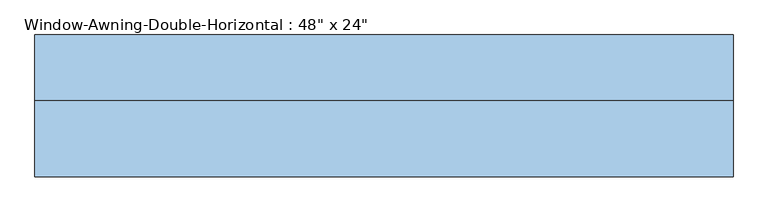
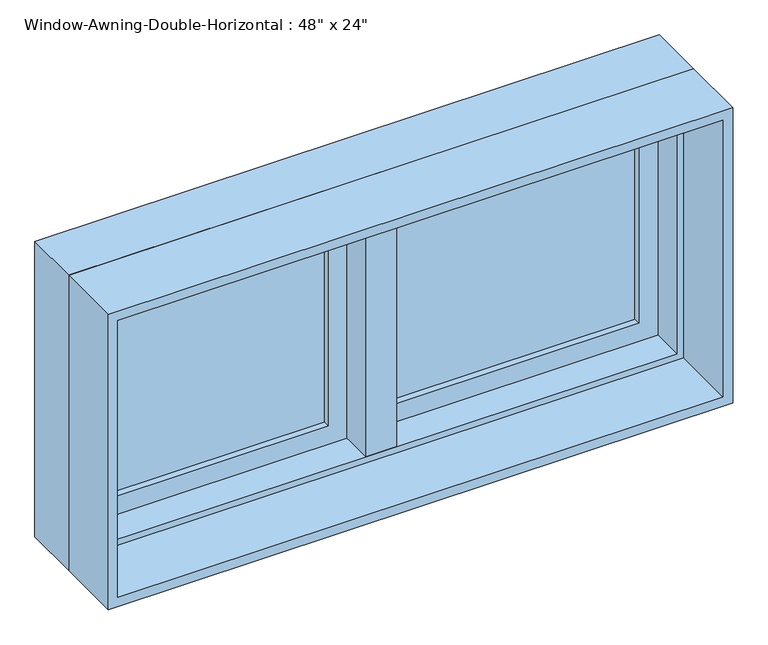
"""IFC4 building model written with IfcOpenShell, lengths in millimetres: window geometry."""

from ifc_helpers import new_model, si_unit, frame, origin, place, context, project, spatial, polyline, outline, extrude, faceted_brep, source, transform, mapped, element, save


def window_133af304(model_context):
    return source(origin(), model_context, "Body", "SolidModel", [
        faceted_brep([(577.85, 82.55, 1492.25), (577.85, 19.05, 1492.25), (-577.85, 19.05, 1492.25), (-577.85, 82.55, 1492.25), (596.9, 133.35, 1511.3), (596.9, 82.55, 1511.3), (-596.9, 82.55, 1511.3), (-596.9, 133.35, 1511.3), (609.6, 19.05, 1524.0), (609.6, 133.35, 1524.0), (-609.6, 133.35, 1524.0), (-609.6, 19.05, 1524.0), (-577.85, 19.05, 946.15), (-577.85, 82.55, 946.15), (-596.9, 82.55, 927.1), (-596.9, 133.35, 927.1), (-609.6, 133.35, 914.4), (-609.6, 19.05, 914.4), (577.85, 19.05, 946.15), (577.85, 82.55, 946.15), (596.9, 82.55, 927.1), (596.9, 133.35, 927.1), (609.6, 133.35, 914.4), (609.6, 19.05, 914.4)], [[[0, 1, 2, 3]], [[4, 5, 6, 7]], [[8, 9, 10, 11]], [[3, 2, 12, 13]], [[7, 6, 14, 15]], [[11, 10, 16, 17]], [[13, 12, 18, 19]], [[15, 14, 20, 21]], [[17, 16, 22, 23]], [[11, 17, 23, 8], [1, 18, 12, 2]], [[19, 18, 1, 0]], [[5, 20, 14, 6], [3, 13, 19, 0]], [[21, 20, 5, 4]], [[23, 22, 9, 8]], [[9, 22, 16, 10], [7, 15, 21, 4]]]),
        extrude(outline(polyline([(1524.0, -609.6), (914.4, -609.6), (914.4, 609.6), (1524.0, 609.6), (1524.0, -609.6)]), holes=[polyline([(1504.95, 590.55), (933.45, 590.55), (933.45, -590.55), (1504.95, -590.55), (1504.95, 590.55)])]), frame((0.0, -114.3, 0.0), z_axis=(0.0, 1.0, 0.0), x_axis=(0.0, 0.0, 1.0)), (0.0, 0.0, 1.0), 133.35),
        extrude(outline(polyline([(927.1, 596.9), (1511.3, 596.9), (1511.3, 9.525), (927.1, 9.525), (927.1, 596.9)]), holes=[polyline([(984.25, 66.675), (1454.15, 66.675), (1454.15, 539.75), (984.25, 539.75), (984.25, 66.675)])]), frame((0.0, 82.55, 0.0), z_axis=(0.0, 1.0, 0.0), x_axis=(0.0, 0.0, 1.0)), (0.0, 0.0, 1.0), 44.45),
        extrude(outline(polyline([(1511.3, -596.9), (927.1, -596.9), (927.1, -9.525), (1511.3, -9.525), (1511.3, -596.9)]), holes=[polyline([(1454.15, -66.675), (984.25, -66.675), (984.25, -539.75), (1454.15, -539.75), (1454.15, -66.675)])]), frame((0.0, 82.55, 0.0), z_axis=(0.0, 1.0, 0.0), x_axis=(0.0, 0.0, 1.0)), (0.0, 0.0, 1.0), 44.45),
        extrude(outline(polyline([(539.75, 114.3), (539.75, 107.95), (66.675, 107.95), (66.675, 114.3), (539.75, 114.3)])), frame((0.0, 0.0, 984.25), z_axis=(0.0, 0.0, 1.0), x_axis=(1.0, 0.0, 0.0)), (0.0, 0.0, 1.0), 469.9),
        extrude(outline(polyline([(66.675, 95.25), (66.675, 101.6), (539.75, 101.6), (539.75, 95.25), (66.675, 95.25)])), frame((0.0, 0.0, 984.25), z_axis=(0.0, 0.0, 1.0), x_axis=(1.0, 0.0, 0.0)), (0.0, 0.0, 1.0), 469.9),
        extrude(outline(polyline([(-66.675, 114.3), (-66.675, 107.95), (-539.75, 107.95), (-539.75, 114.3), (-66.675, 114.3)])), frame((0.0, 0.0, 984.25), z_axis=(0.0, 0.0, 1.0), x_axis=(1.0, 0.0, 0.0)), (0.0, 0.0, 1.0), 469.9),
        extrude(outline(polyline([(-539.75, 95.25), (-539.75, 101.6), (-66.675, 101.6), (-66.675, 95.25), (-539.75, 95.25)])), frame((0.0, 0.0, 984.25), z_axis=(0.0, 0.0, 1.0), x_axis=(1.0, 0.0, 0.0)), (0.0, 0.0, 1.0), 469.9),
        faceted_brep([(9.525, 133.35, 1511.3), (-9.525, 133.35, 1511.3), (-9.525, 82.55, 1511.3), (9.525, 82.55, 1511.3), (9.525, 133.35, 927.1), (9.525, 82.55, 927.1), (-9.525, 82.55, 927.1), (-9.525, 133.35, 927.1), (-9.525, 82.55, 946.15), (-9.525, 82.55, 1492.25), (-30.1625, 82.55, 946.15), (-30.1625, 82.55, 1492.25), (-30.1625, 19.05, 946.15), (-30.1625, 19.05, 1492.25), (30.1625, 19.05, 946.15), (30.1625, 19.05, 1492.25), (30.1625, 82.55, 946.15), (30.1625, 82.55, 1492.25), (9.525, 82.55, 946.15), (9.525, 82.55, 1492.25)], [[[0, 1, 2, 3]], [[4, 5, 6, 7]], [[1, 0, 4, 7]], [[2, 1, 7, 6, 8, 9]], [[9, 8, 10, 11]], [[11, 10, 12, 13]], [[13, 12, 14, 15]], [[15, 14, 16, 17]], [[17, 16, 18, 19]], [[0, 3, 19, 18, 5, 4]], [[18, 8, 6, 5]], [[9, 19, 3, 2]], [[8, 18, 16, 14, 12, 10]], [[19, 9, 11, 13, 15, 17]]]),
    ])


if __name__ == "__main__":
    model = new_model("IFC4")
    model_context = context("Model", 3, world=origin())
    ifc_project = project(units=[si_unit("LENGTHUNIT", "METRE", prefix="MILLI")], contexts=[model_context])
    site = spatial("IfcSite", under=ifc_project)
    building = spatial("IfcBuilding", under=site)
    placement = place(None, origin())
    window_shape = window_133af304(model_context)
    element("IfcWindow", 1, ObjectType="Window-Awning-Double-Horizontal : 48\" x 24\"", at=placement, inside=building, context=model_context, shape_type="MappedRepresentation", body=[
        mapped(window_shape, transform((0.0, 0.0, 0.0), x_axis=(1.0, 0.0, 0.0), y_axis=(0.0, 1.0, 0.0), z_axis=(0.0, 0.0, 1.0))),
    ])
    save(model, "model.ifc")

# Revit data of these elements
# Type "Window-Awning-Double-Horizontal : 48\" x 24\""
#   Type Mark = "20"
#   Fire Rating = "0.5h"
#   Assembly Code = "B2020100"
#   Analytic Construction = "Double glazing - domestic"
#   Window Inset [instance default] = 0' - 0"
#   Wall Thickness [instance default] = 0' - 6"
#   Interior Wall Closure [instance default] = 0' - 2 1/4"
#   Half Width = 2' - 0"
#   Visual Light Transmittance = 0.81
#   Thermal Resistance (R) = 1.8146 (h·ft²·°F)/BTU
#   Solar Heat Gain Coefficient = 0.76
#   Rough Width = 4' - 0 1/2"
#   Rough Height = 2' - 0 1/2"
#   Height = 2' - 0"
#   Heat Transfer Coefficient (U) = 0.5511 BTU/(h·ft²·°F)
#   Frame Extension [instance default] = 0' - 0 1/4"
#   Exterior Wall Closure [instance default] = 0' - 1 1/4"
#   Extension Jamb [instance default] = 0' - 2 1/4"
#   Default Sill Height = 3' - 0"
#   Width = 4' - 0"
#   Muntin Visibility = yes
#   Interior Trim Visibility [instance default] = yes
#   Exterior Trim Visibility [instance default] = yes
#   Extension Jamb Visibility [instance default] = yes
#   Interior Trim Material = Wood - Stained
#   Muntin Pattern = Muntin Pattern_2x2 : Muntin Pattern_2x2
#   Interior Trim = Trim-Window-Interior-Flat : Picture Frame
#   Interior Frame Material = Wood - Stained
#   Glass Panel Material = Glass
#   Exterior Trim Material = Clad - White
#   Exterior Trim = Trim-Window-Exterior-Flat : with Sill
#   Exterior Frame Material = Clad - White
#   Wall Closure = (empty or 0)
# Element 1 (IfcWindow, "Window-Awning-Double-Horizontal : 48\" x 24\"")
#   Wall Thickness = 0' - 9"
#   Extension Jamb = 0' - 5 1/4"
#   Materials on its faces: "Wood - Stained", "Glass", "Clad - White"
# Materials
#   "Wood - Stained": class "Wood", colour RGB 224 178 126, transparency 0, Cost = 0
#   "Glass": class "Glass", colour RGB 0 128 192, transparency 0.75, Description = "Soda Lime Glass", Cost = 0
#   "Clad - White": class "Wood", colour RGB 242 242 238, transparency 0, Cost = 0
